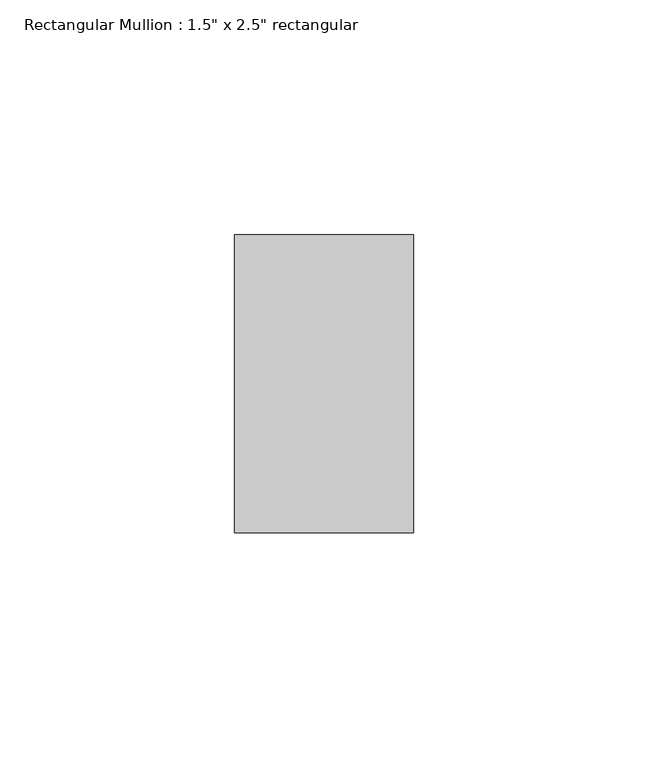
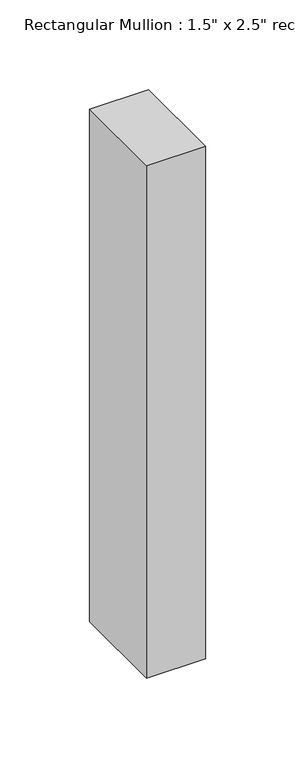
"""IFC4 building model written with IfcOpenShell, lengths in millimetres: member geometry."""

from ifc_helpers import new_model, si_unit, frame, origin, place, context, project, spatial, polyline, outline, extrude, source, transform, mapped, element, save


def member_07b5019b(model_context):
    return source(origin(), model_context, "Body", "SweptSolid", [
        extrude(outline(polyline([(0.0, 31.75), (0.0, -31.75), (-38.1, -31.75), (-38.1, 31.75), (0.0, 31.75)])), frame((0.0, 0.0, -349.25), z_axis=(0.0, 0.0, 1.0), x_axis=(1.0, 0.0, 0.0)), (0.0, 0.0, 1.0), 349.25),
    ])


if __name__ == "__main__":
    model = new_model("IFC4")
    model_context = context("Model", 3, world=origin())
    ifc_project = project(units=[si_unit("LENGTHUNIT", "METRE", prefix="MILLI")], contexts=[model_context])
    site = spatial("IfcSite", under=ifc_project)
    building = spatial("IfcBuilding", under=site)
    placement = place(None, origin())
    member_shape = member_07b5019b(model_context)
    element("IfcMember", 1, ObjectType="Rectangular Mullion : 1.5\" x 2.5\" rectangular", at=placement, inside=building, context=model_context, shape_type="MappedRepresentation", body=[
        mapped(member_shape, transform((0.0, 0.0, 0.0), x_axis=(1.0, 0.0, 0.0), y_axis=(0.0, 1.0, 0.0), z_axis=(0.0, 0.0, 1.0))),
    ])
    save(model, "model.ifc")

# Revit data of these elements
# Type "Rectangular Mullion : 1.5\" x 2.5\" rectangular"
#   built-in parameter 1007304 = 0.208333 (stored number, unit not read)
#   built-in parameter 1007301 = 0.0625 (stored number, unit not read)
#   built-in parameter 1007300 = 0.0625 (stored number, unit not read)
# Element 1 (IfcMember, "Rectangular Mullion : 1.5\" x 2.5\" rectangular")
#   Materials on its faces: "Damp-proofing"
# Materials
#   "Damp-proofing": class "Generic", colour RGB 127 127 127, transparency 0, Description = "Damp-proofing", Cost = 0
